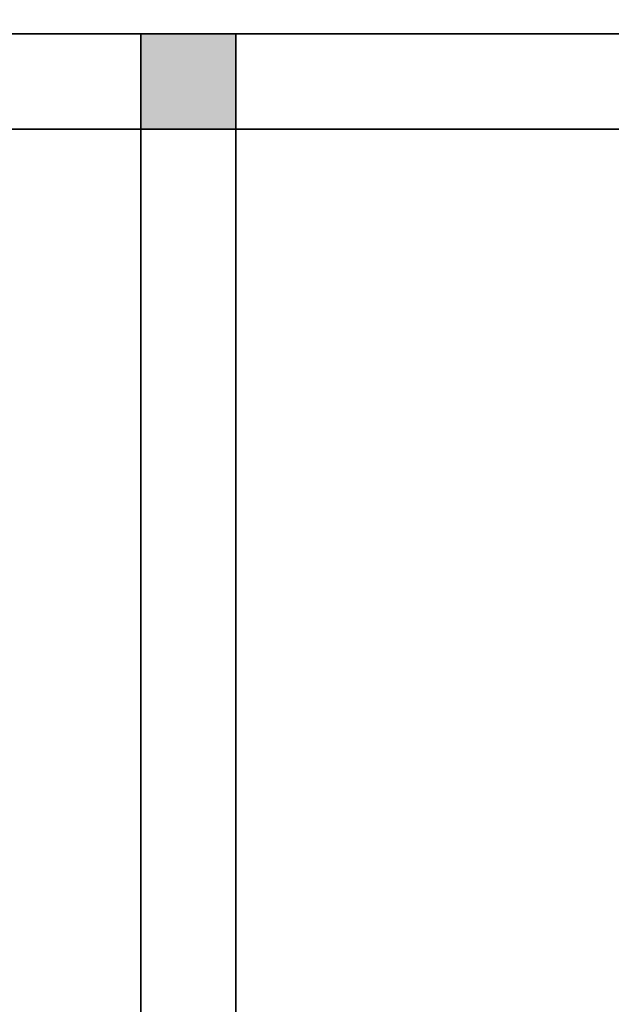
# Model space of a CAD drawing. Units: inches. Extents: x -36302355 to 648, y -221479757 to 75.
# Tile 31 of 37: x 227 to 283, y -67 to 26. Entities that reach past the tile are written whole.
import ezdxf

# ---------------------------------------------------------------- set-up
doc = ezdxf.new("R2010")
doc.units = ezdxf.units.IN
doc.header["$MEASUREMENT"] = 0
for name, color, linetype, lineweight in [('A-ANNO-DIMS', 2, 'Continuous', 18), ('A-COLS-PATT', 242, 'Continuous', 13), ('A-WALL', 7, 'Continuous', 35)]:
    doc.layers.add(name, color=color, linetype=linetype, lineweight=lineweight)
doc.styles.get("Standard").update_dxf_attribs({"font": 'arial.ttf'})
doc.dimstyles.get("Standard").update_dxf_attribs({"dimtxt": 0.18, "dimasz": 0.18, "dimexe": 0.18, "dimexo": 0.0625, "dimgap": 0.09, "dimtad": 0, "dimtih": 1, "dimtoh": 1, "dimdec": 0, "dimzin": 0, "dimdsep": 46, "dimlunit": 3, "dimtxsty": 'Standard', "dimcen": 0.09, "dimadec": 0, "dimazin": 0, "dimtfac": 1, "dimtdec": 0, "dimtofl": 0, "dimtmove": 0, "dimatfit": 3, "dimfxl": 1, "dimtolj": 1, "dimtzin": 0, "dimarcsym": 0})

# ---------------------------------------------------------------- blocks, each defined once
blk = doc.blocks.new('*D4')
at = {"layer": 'A-ANNO-DIMS', "color": 0, "lineweight": -2, "transparency": 16777216}
for p, q in [((145.197, 25.043), (145.197, 71.11)), ((145.377, 70.93), (364.803, 70.93)), ((605.017, 70.93), (385.59, 70.93)), ((605.197, 25.043), (605.197, 71.11))]:
    blk.add_line(p, q, dxfattribs=at)
at = {"layer": 'A-ANNO-DIMS', "color": 0, "transparency": 16777216}
for points in [[(145.377, 70.96), (145.377, 70.9), (145.197, 70.93)], [(605.017, 70.96), (605.017, 70.9), (605.197, 70.93)]]:
    blk.add_solid(points, dxfattribs=at)
at = {"layer": 'Defpoints', "color": 0, "transparency": 16777216}
for p in [(605.197, 70.93), (145.197, 24.981), (605.197, 24.981)]:
    blk.add_point(p, dxfattribs=at)
at = {"layer": 'A-ANNO-DIMS', "color": 0, "transparency": 16777216, "insert": (375.197, 70.93), "char_height": 6, "attachment_point": 5}
blk.add_mtext('\\A1;38\'-4"', dxfattribs=at)

msp = doc.modelspace()

# ---------------------------------------------------------------- hatches: boundary and pattern name
at = {"layer": 'A-COLS-PATT'}
h = msp.add_hatch(color=256, dxfattribs=at)
h.dxf.hatch_style = 1
h.paths.add_polyline_path([(145.197, 24.981), (145.197, 15.981), (154.197, 15.981), (154.197, 24.981)])
h.paths.add_polyline_path([(247.197, 15.981), (247.197, 24.981), (238.197, 24.981), (238.197, 15.981)])
h.paths.add_polyline_path([(387.635, 15.981), (395.697, 15.981), (395.697, 24.981), (387.635, 24.981)])
h.paths.add_polyline_path([(451.263, 24.981), (443.697, 24.981), (443.697, 15.981), (451.263, 15.981)])
h.paths.add_polyline_path([(596.197, 15.981), (605.197, 15.981), (605.197, 24.981), (596.197, 24.981)])
h.paths.add_polyline_path([(238.197, -122.019), (238.197, -131.019), (247.197, -131.019), (247.197, -122.019)])
h.paths.add_polyline_path([(395.697, -122.019), (387.459, -122.019), (387.459, -131.019), (395.697, -131.019)])
h.paths.add_polyline_path([(448.197, -131.019), (453.734, -131.019), (453.734, -122.019), (443.697, -122.019), (443.697, -131.019)])
h.paths.add_polyline_path([(596.197, -131.019), (605.197, -131.019), (605.197, -122.019), (596.197, -122.019)])
h.paths.add_polyline_path([(145.197, -176.971), (154.197, -176.971), (154.197, -167.019), (145.197, -167.019)])
h.paths.add_polyline_path([(314.197, -176.971), (323.197, -176.971), (323.197, -167.019), (314.197, -167.019)])
h.paths.add_polyline_path([(154.197, -314.019), (154.197, -309.519), (145.197, -309.519), (145.197, -314.019)])
h.paths.add_polyline_path([(314.197, -309.519), (314.197, -318.519), (323.197, -318.519), (323.197, -309.519)])
h.paths.add_polyline_path([(448.197, -277.019), (443.697, -277.019), (443.697, -286.019), (448.197, -286.019)])
h.paths.add_polyline_path([(283.197, -370.019), (274.197, -370.019), (274.197, -379.019), (283.197, -379.019), (283.197, -374.519)])
h.paths.add_polyline_path([(154.197, -370.019), (145.197, -370.019), (145.197, -379.019), (154.197, -379.019)])
h.paths.add_polyline_path([(443.197, -374.519), (443.197, -379.019), (452.197, -379.019), (452.197, -374.519)])
h.paths.add_polyline_path([(145.197, -580.019), (154.197, -580.019), (154.197, -571.019), (145.197, -571.019)])
h.paths.add_polyline_path([(274.197, -571.019), (274.197, -580.019), (283.197, -580.019), (283.197, -571.019)])
h.paths.add_polyline_path([(443.197, -580.019), (452.197, -580.019), (452.197, -571.019), (443.197, -571.019)])

# ---------------------------------------------------------------- linework, layer by layer
at = {"layer": 'A-WALL'}
for p, q in [((145.197, 24.981), (605.197, 24.981)), ((238.197, 24.981), (238.197, -131.019)), ((247.197, 24.981), (247.197, -131.019)), ((145.197, 15.981), (605.197, 15.981))]:
    msp.add_line(p, q, dxfattribs=at)

# ---------------------------------------------------------------- dimensions: what is measured, and where the dimension line sits
at = {"layer": 'A-ANNO-DIMS'}
dim = msp.add_linear_dim(base=(605.197, 70.93), p1=(145.197, 24.981), p2=(605.197, 24.981), dimstyle='Standard', override={"dimtxt": 6, "dimclrd": 0, "dimclre": 0, "dimclrt": 0}, dxfattribs=at)
dim.commit()
dim.dimension.update_dxf_attribs({"geometry": '*D4', "text_midpoint": (375.197, 70.93)})

doc.saveas('drawing.dxf')
